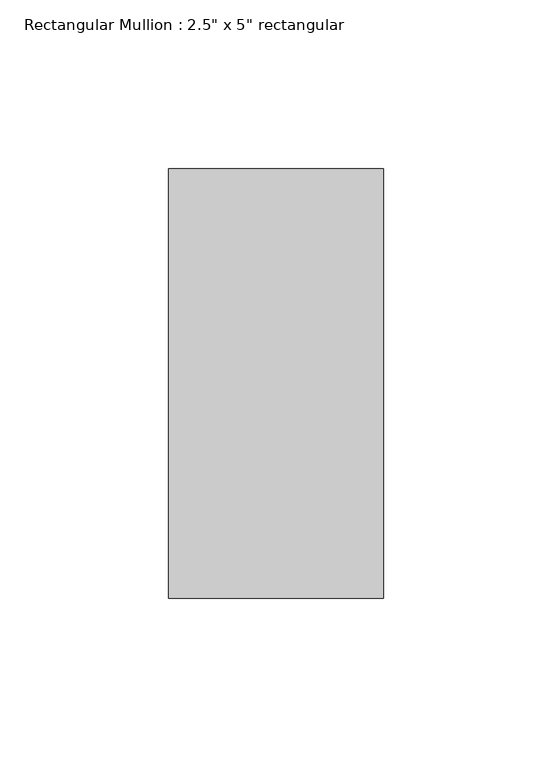
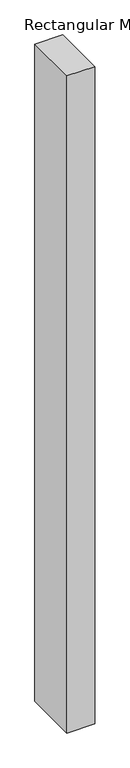
"""IFC4 building model written with IfcOpenShell, lengths in millimetres: member geometry."""

from ifc_helpers import new_model, si_unit, frame, origin, place, context, project, spatial, polyline, outline, extrude, source, transform, mapped, element, save


def member_9a58012a(model_context):
    return source(origin(), model_context, "Body", "SweptSolid", [
        extrude(outline(polyline([(31.75, 63.5), (31.75, -63.5), (-31.75, -63.5), (-31.75, 63.5), (31.75, 63.5)])), frame((0.0, 0.0, -1589.6963029), z_axis=(0.0, 0.0, 1.0), x_axis=(1.0, 0.0, 0.0)), (0.0, 0.0, 1.0), 1589.6963029),
    ])


if __name__ == "__main__":
    model = new_model("IFC4")
    model_context = context("Model", 3, world=origin())
    ifc_project = project(units=[si_unit("LENGTHUNIT", "METRE", prefix="MILLI")], contexts=[model_context])
    site = spatial("IfcSite", under=ifc_project)
    building = spatial("IfcBuilding", under=site)
    placement = place(None, origin())
    member_shape = member_9a58012a(model_context)
    element("IfcMember", 1, ObjectType="Rectangular Mullion : 2.5\" x 5\" rectangular", at=placement, inside=building, context=model_context, shape_type="MappedRepresentation", body=[
        mapped(member_shape, transform((0.0, 0.0, 0.0), x_axis=(1.0, 0.0, 0.0), y_axis=(0.0, 1.0, 0.0), z_axis=(0.0, 0.0, 1.0))),
    ])
    save(model, "model.ifc")

# Revit data of these elements
# Type "Rectangular Mullion : 2.5\" x 5\" rectangular"
#   built-in parameter 1007304 = 0.416667 (stored number, unit not read)
#   built-in parameter 1007301 = 0.104167 (stored number, unit not read)
#   built-in parameter 1007300 = 0.104167 (stored number, unit not read)
# Element 1 (IfcMember, "Rectangular Mullion : 2.5\" x 5\" rectangular")
#   Materials on its faces: "Aluminum"
# Materials
#   "Aluminum": class "Metal", colour RGB 247 247 247, transparency 0, Description = "Aluminum 6061", Cost = 0
